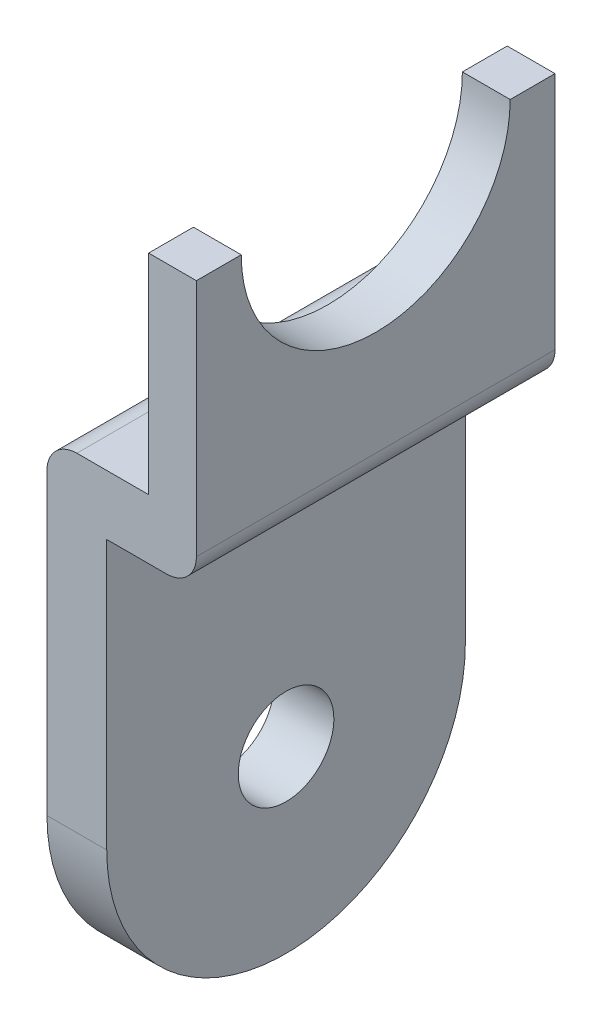
SolidWorks part; units mm, degrees
material "Plain Carbon Steel"
ref_plane "Front Plane" through (0, 0, 0) normal (0, 0, 1) x (1, 0, 0)
ref_plane "Top Plane" through (0, 0, 0) normal (0, 1, 0) x (1, 0, 0)
ref_plane "Right Plane" through (0, 0, 0) normal (1, 0, 0) x (0, 0, -1)
sketch "Clip Profile Sketch" plane through (0, 0, 0) normal (0, 0, 1) x (1, 0, 0)
  line L0 (0, -11) -> (0, 0)
  line L1 (0, 0) -> (3.4, 0)
  line L2 (3.4, 0) -> (3.4, 7)
  line L3 (3.4, 7) -> (5, 7)
  line L4 (5, 7) -> (5, -2)
  line L5 (5, -2) -> (2, -2)
  line L6 (2, -2) -> (2, -11)
  line L7 (2, -11) -> (0, -11)
  point P3 (4.2, 7)
  dimension "D1" = 3.4
  dimension "D2" = 2
  dimension "D3" = 1.6
  dimension "D4" = 2
  dimension "D5" = 9
  dimension "D6" = 18
extrude "Clip Body" add sketch "Clip Profile Sketch" along normal mid plane 12
sketch "Rounded Tab Sketch" plane through (2, 0, 0) normal (1, 0, 0) x (0, 0, -1)
  line L0 (-6, -11) -> (6, -11) construction
  circle A0 centre (0, -11) radius 6
extrude "Rounded Tab" add sketch "Rounded Tab Sketch" against normal up to surface (2 mm away) up to face at (0, -5.5, 0)
sketch "Saddle Cut Sketch" plane through (5, 0, 0) normal (1, 0, 0) x (0, 0, -1)
  line L0 (-6, 7) -> (6, 7) construction
  line L1 (-4.5, 7) -> (4.5, 7)
  line L2 (6, -2) -> (6, 7) construction
  arc A0 (-4.5, 7) -> (4.5, 7) centre (0, 7) ccw
  dimension "D1" = 4.5
  dimension "D2" = 1.5
  dimension "D3" = 1.5
extrude "Saddle Cut" cut sketch "Saddle Cut Sketch" against normal up to next
sketch "Pivot Hole Sketch" plane through (2, 0, 0) normal (1, 0, 0) x (0, 0, -1)
  circle A0 centre (0, -11) radius 1.6
  point P0 (0, -11)
  dimension "D1" = 3.2
extrude "Pivot Hole Ø3.2" cut sketch "Pivot Hole Sketch" against normal up to next
fillet "Edge Fillets R1" radius 1 2 edges at (5, -2, 0) (0, 0, 0)
